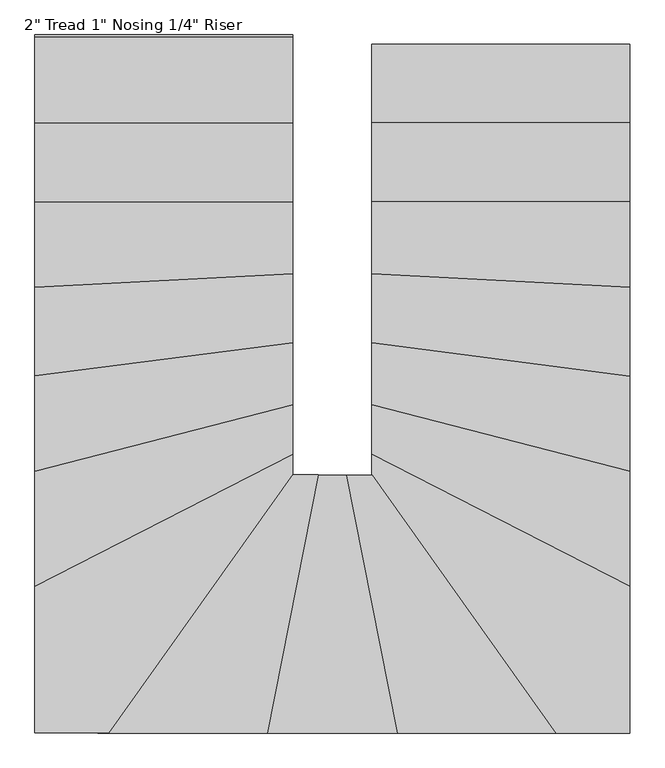
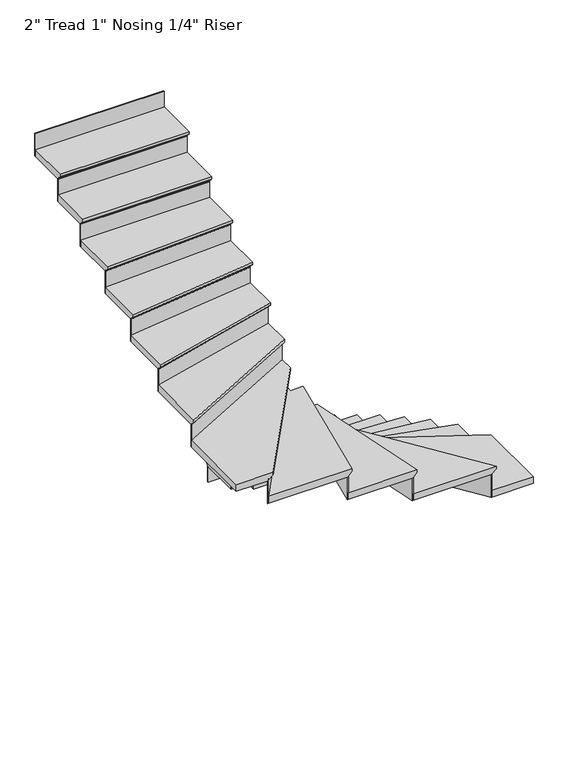
"""IFC4 building model written with IfcOpenShell, lengths in millimetres: stair flight geometry."""

from ifc_helpers import new_model, si_unit, origin, place, context, project, spatial, faceted_brep, source, transform, mapped, element, save


def stair_flight_703d0d0a(model_context):
    return source(origin(), model_context, "Body", "Brep", [
        faceted_brep([(-4178.4918623, -2804.4089531, 150.2833333), (-4178.4918623, -2804.4089531, 169.3333333), (-3264.0918623, -2804.4089531, 169.3333333), (-3264.0918623, -2804.4089531, 150.2833333), (-4178.4918623, -2829.8089531, 124.8833333), (-3264.0918623, -2829.8089531, 124.8833333), (-4178.4918623, -3109.2089531, 169.3333333), (-3264.0918623, -3109.2089531, 169.3333333), (-3264.0918623, -2829.8089531, 118.5333333), (-3264.0918623, -3109.2089531, 118.5333333), (-4178.4918623, -3109.2089531, 118.5333333), (-4178.4918623, -2829.8089531, 118.5333333)], [[[0, 1, 2, 3]], [[4, 0, 3, 5]], [[2, 1, 6, 7]], [[8, 9, 10, 11]], [[2, 7, 9, 8, 5, 3]], [[8, 11, 4, 5]], [[6, 1, 0, 4, 11, 10]], [[7, 6, 10, 9]]]),
        faceted_brep([(-4178.4918623, -2829.8089531, 118.5333333), (-4178.4918623, -2829.8089531, 0.0), (-4178.4918623, -2836.1589531, 0.0), (-4178.4918623, -2836.1589531, 118.5333333), (-3264.0918623, -2829.8089531, 118.5333333), (-3264.0918623, -2836.1589531, 118.5333333), (-3264.0918623, -2836.1589531, 0.0), (-3264.0918623, -2829.8089531, 0.0)], [[[0, 1, 2, 3]], [[4, 5, 6, 7]], [[1, 0, 4, 7]], [[2, 1, 7, 6]], [[3, 2, 6, 5]], [[0, 3, 5, 4]]]),
        faceted_brep([(-4178.4918623, -3109.2089531, 287.8666667), (-4178.4918623, -3109.2089531, 118.5333333), (-4178.4918623, -3115.5589531, 118.5333333), (-4178.4918623, -3115.5589531, 287.8666667), (-3264.0918623, -3109.2089531, 287.8666667), (-3264.0918623, -3115.5589531, 287.8666667), (-3264.0918623, -3115.5589531, 118.5333333), (-3264.0918623, -3109.2089531, 118.5333333)], [[[0, 1, 2, 3]], [[4, 5, 6, 7]], [[1, 0, 4, 7]], [[2, 1, 7, 6]], [[3, 2, 6, 5]], [[0, 3, 5, 4]]]),
        faceted_brep([(-3264.0918623, -3083.8089531, 338.6666667), (-4178.4918623, -3083.8089531, 338.6666667), (-4178.4918623, -3388.6089531, 338.6666667), (-3264.0918623, -3388.6089531, 338.6666667), (-3264.0918623, -3109.2089531, 287.8666667), (-3264.0918623, -3388.6089531, 287.8666667), (-4178.4918623, -3388.6089531, 287.8666667), (-4178.4918623, -3109.2089531, 287.8666667), (-3264.0918623, -3109.2089531, 294.2166667), (-3264.0918623, -3083.8089531, 319.6166667), (-4178.4918623, -3109.2089531, 294.2166667), (-4178.4918623, -3083.8089531, 319.6166667)], [[[0, 1, 2, 3]], [[4, 5, 6, 7]], [[0, 3, 5, 4, 8, 9]], [[4, 7, 10, 8]], [[2, 1, 11, 10, 7, 6]], [[3, 2, 6, 5]], [[11, 1, 0, 9]], [[10, 11, 9, 8]]]),
        faceted_brep([(-4178.4918623, -3388.6089531, 457.2), (-4178.4918623, -3388.6089531, 287.8666667), (-4178.4918623, -3394.9589531, 287.8666667), (-4178.4918623, -3394.9589531, 457.2), (-3264.0918623, -3388.6089531, 457.2), (-3264.0918623, -3394.9589531, 457.2), (-3264.0918623, -3394.9589531, 287.8666667), (-3264.0918623, -3388.6089531, 287.8666667)], [[[0, 1, 2, 3]], [[4, 5, 6, 7]], [[1, 0, 4, 7]], [[2, 1, 7, 6]], [[3, 2, 6, 5]], [[0, 3, 5, 4]]]),
        faceted_brep([(-3264.0918623, -3363.2089531, 508.0), (-4178.4918623, -3363.2089531, 508.0), (-4178.4918623, -3644.2761146, 508.0), (-3264.0918623, -3691.810385, 508.0), (-3264.0918623, -3388.6089531, 457.2), (-3264.0918623, -3691.810385, 457.2), (-4178.4918623, -3644.2761146, 457.2), (-4178.4918623, -3388.6089531, 457.2), (-3264.0918623, -3388.6089531, 463.55), (-3264.0918623, -3363.2089531, 488.95), (-4178.4918623, -3388.6089531, 463.55), (-4178.4918623, -3363.2089531, 488.95)], [[[0, 1, 2, 3]], [[4, 5, 6, 7]], [[0, 3, 5, 4, 8, 9]], [[4, 7, 10, 8]], [[2, 1, 11, 10, 7, 6]], [[3, 2, 6, 5]], [[11, 1, 0, 9]], [[10, 11, 9, 8]]]),
        faceted_brep([(-4178.4918623, -3644.2761146, 626.5333333), (-4178.4918623, -3644.2761146, 457.2), (-4178.4918623, -3650.6346887, 457.2), (-4178.4918623, -3650.6346887, 626.5333333), (-3264.0918623, -3691.810385, 626.5333333), (-3264.0918623, -3698.1689591, 626.5333333), (-3264.0918623, -3698.1689591, 457.2), (-3264.0918623, -3691.810385, 457.2)], [[[0, 1, 2, 3]], [[4, 5, 6, 7]], [[1, 0, 4, 7]], [[2, 1, 7, 6]], [[3, 2, 6, 5]], [[0, 3, 5, 4]]]),
        faceted_brep([(-3264.0918623, -3666.3760883, 677.3333333), (-4178.4918623, -3618.8418179, 677.3333333), (-4178.4918623, -3888.4428144, 677.3333333), (-3264.0918623, -4006.798866, 677.3333333), (-3264.0918623, -3691.810385, 626.5333333), (-3264.0918623, -4006.798866, 626.5333333), (-4178.4918623, -3888.4428144, 626.5333333), (-4178.4918623, -3644.2761146, 626.5333333), (-3264.0918623, -3691.810385, 632.8833333), (-3264.0918623, -3666.3760883, 658.2833333), (-4178.4918623, -3644.2761146, 632.8833333), (-4178.4918623, -3618.8418179, 658.2833333)], [[[0, 1, 2, 3]], [[4, 5, 6, 7]], [[0, 3, 5, 4, 8, 9]], [[4, 7, 10, 8]], [[2, 1, 11, 10, 7, 6]], [[3, 2, 6, 5]], [[11, 1, 0, 9]], [[10, 11, 9, 8]]]),
        faceted_brep([(-4178.4918623, -3888.4428144, 795.8666667), (-4178.4918623, -3888.4428144, 626.5333333), (-4178.4918623, -3894.8457862, 626.5333333), (-4178.4918623, -3894.8457862, 795.8666667), (-3264.0918623, -4006.798866, 795.8666667), (-3264.0918623, -4013.2018378, 795.8666667), (-3264.0918623, -4013.2018378, 626.5333333), (-3264.0918623, -4006.798866, 626.5333333)], [[[0, 1, 2, 3]], [[4, 5, 6, 7]], [[1, 0, 4, 7]], [[2, 1, 7, 6]], [[3, 2, 6, 5]], [[0, 3, 5, 4]]]),
        faceted_brep([(-3264.0918623, -3981.1869789, 846.6666667), (-4178.4918623, -3862.8309273, 846.6666667), (-4178.4918623, -4110.0700369, 846.6666667), (-3264.0918623, -4345.2004843, 846.6666667), (-3264.0918623, -4006.798866, 795.8666667), (-3264.0918623, -4345.2004843, 795.8666667), (-4178.4918623, -4110.0700369, 795.8666667), (-4178.4918623, -3888.4428144, 795.8666667), (-3264.0918623, -4006.798866, 802.2166667), (-3264.0918623, -3981.1869789, 827.6166667), (-4178.4918623, -3888.4428144, 802.2166667), (-4178.4918623, -3862.8309273, 827.6166667)], [[[0, 1, 2, 3]], [[4, 5, 6, 7]], [[0, 3, 5, 4, 8, 9]], [[4, 7, 10, 8]], [[2, 1, 11, 10, 7, 6]], [[3, 2, 6, 5]], [[11, 1, 0, 9]], [[10, 11, 9, 8]]]),
        faceted_brep([(-4178.4918623, -4110.0700369, 965.2), (-4178.4918623, -4110.0700369, 795.8666667), (-4178.4918623, -4116.6266137, 795.8666667), (-4178.4918623, -4116.6266137, 965.2), (-3264.0918623, -4345.2004843, 965.2), (-3264.0918623, -4351.7570611, 965.2), (-3264.0918623, -4351.7570611, 795.8666667), (-3264.0918623, -4345.2004843, 795.8666667)], [[[0, 1, 2, 3]], [[4, 5, 6, 7]], [[1, 0, 4, 7]], [[2, 1, 7, 6]], [[3, 2, 6, 5]], [[0, 3, 5, 4]]]),
        faceted_brep([(-3264.0918623, -4318.9741768, 1016.0), (-4178.4918623, -4083.8437294, 1016.0), (-4178.4918623, -4286.4166729, 1016.0), (-3264.0918623, -4755.2412943, 1016.0), (-3264.0918623, -4345.2004843, 965.2), (-3264.0918623, -4755.2412943, 965.2), (-4178.4918623, -4286.4166729, 965.2), (-4178.4918623, -4110.0700369, 965.2), (-3264.0918623, -4345.2004843, 971.55), (-3264.0918623, -4318.9741768, 996.95), (-4178.4918623, -4110.0700369, 971.55), (-4178.4918623, -4083.8437294, 996.95)], [[[0, 1, 2, 3]], [[4, 5, 6, 7]], [[0, 3, 5, 4, 8, 9]], [[4, 7, 10, 8]], [[2, 1, 11, 10, 7, 6]], [[3, 2, 6, 5]], [[11, 1, 0, 9]], [[10, 11, 9, 8]]]),
        faceted_brep([(-4178.4918623, -4286.4166729, 1134.5333333), (-4178.4918623, -4286.4166729, 965.2), (-4178.4918623, -4293.5526561, 965.2), (-4178.4918623, -4293.5526561, 1134.5333333), (-3264.0918623, -4755.2412943, 1134.5333333), (-3264.0918623, -4762.3772774, 1134.5333333), (-3264.0918623, -4762.3772774, 965.2), (-3264.0918623, -4755.2412943, 965.2)], [[[0, 1, 2, 3]], [[4, 5, 6, 7]], [[1, 0, 4, 7]], [[2, 1, 7, 6]], [[3, 2, 6, 5]], [[0, 3, 5, 4]]]),
        faceted_brep([(-3557.772996, -5246.540645, 1185.3333333), (-3264.0918623, -5246.540645, 1185.3333333), (-3264.0918623, -4726.6973617, 1185.3333333), (-4178.4918623, -4257.8727404, 1185.3333333), (-4178.4918623, -4332.140645, 1185.3333333), (-4208.0469452, -4332.140645, 1185.3333333), (-3264.0918623, -5246.540645, 1134.5333333), (-3557.772996, -5246.540645, 1134.5333333), (-4208.0469452, -4332.140645, 1134.5333333), (-4178.4918623, -4332.140645, 1134.5333333), (-4178.4918623, -4286.4166729, 1134.5333333), (-3264.0918623, -4755.2412943, 1134.5333333), (-3264.0918623, -4755.2412943, 1140.8833333), (-3264.0918623, -4726.6973617, 1166.2833333), (-4178.4918623, -4286.4166729, 1140.8833333), (-4178.4918623, -4257.8727404, 1166.2833333)], [[[0, 1, 2, 3, 4, 5]], [[6, 7, 8, 9, 10, 11]], [[1, 0, 7, 6]], [[2, 1, 6, 11, 12, 13]], [[11, 10, 14, 12]], [[4, 3, 15, 14, 10, 9]], [[5, 4, 9, 8]], [[0, 5, 8, 7]], [[15, 3, 2, 13]], [[14, 15, 13, 12]]]),
        faceted_brep([(-4208.0469452, -4332.140645, 1303.8666667), (-4208.0469452, -4332.140645, 1134.5333333), (-4215.83892, -4332.140645, 1134.5333333), (-4215.83892, -4332.140645, 1303.8666667), (-3557.772996, -5246.540645, 1303.8666667), (-3565.5649708, -5246.540645, 1303.8666667), (-3565.5649708, -5246.540645, 1134.5333333), (-3557.772996, -5246.540645, 1134.5333333)], [[[0, 1, 2, 3]], [[4, 5, 6, 7]], [[1, 0, 4, 7]], [[2, 1, 7, 6]], [[3, 2, 6, 5]], [[0, 3, 5, 4]]]),
        faceted_brep([(-3526.6050968, -5246.540645, 1354.6666667), (-4176.879046, -4332.140645, 1354.6666667), (-4294.5010322, -4332.140645, 1354.6666667), (-4114.2601759, -5246.540645, 1354.6666667), (-3557.772996, -5246.540645, 1303.8666667), (-4114.2601759, -5246.540645, 1303.8666667), (-4294.5010322, -4332.140645, 1303.8666667), (-4208.0469452, -4332.140645, 1303.8666667), (-3557.772996, -5246.540645, 1310.2166667), (-3526.6050968, -5246.540645, 1335.6166667), (-4208.0469452, -4332.140645, 1310.2166667), (-4176.879046, -4332.140645, 1335.6166667)], [[[0, 1, 2, 3]], [[4, 5, 6, 7]], [[0, 3, 5, 4, 8, 9]], [[4, 7, 10, 8]], [[2, 1, 11, 10, 7, 6]], [[3, 2, 6, 5]], [[11, 1, 0, 9]], [[10, 11, 9, 8]]]),
        faceted_brep([(-4294.5010322, -4332.140645, 1473.2), (-4294.5010322, -4332.140645, 1303.8666667), (-4300.9732177, -4332.140645, 1303.8666667), (-4300.9732177, -4332.140645, 1473.2), (-4114.2601759, -5246.540645, 1473.2), (-4120.7323613, -5246.540645, 1473.2), (-4120.7323613, -5246.540645, 1303.8666667), (-4114.2601759, -5246.540645, 1303.8666667)], [[[0, 1, 2, 3]], [[4, 5, 6, 7]], [[1, 0, 4, 7]], [[2, 1, 7, 6]], [[3, 2, 6, 5]], [[0, 3, 5, 4]]]),
        faceted_brep([(-4088.3714342, -5246.540645, 1524.0), (-4268.6122905, -4332.140645, 1524.0), (-4393.6601759, -4332.140645, 1524.0), (-4573.9010322, -5246.540645, 1524.0), (-4114.2601759, -5246.540645, 1473.2), (-4573.9010322, -5246.540645, 1473.2), (-4393.6601759, -4332.140645, 1473.2), (-4294.5010322, -4332.140645, 1473.2), (-4114.2601759, -5246.540645, 1479.55), (-4088.3714342, -5246.540645, 1504.95), (-4294.5010322, -4332.140645, 1479.55), (-4268.6122905, -4332.140645, 1504.95)], [[[0, 1, 2, 3]], [[4, 5, 6, 7]], [[0, 3, 5, 4, 8, 9]], [[4, 7, 10, 8]], [[2, 1, 11, 10, 7, 6]], [[3, 2, 6, 5]], [[11, 1, 0, 9]], [[10, 11, 9, 8]]]),
        faceted_brep([(-4393.6601759, -4332.140645, 1642.5333333), (-4393.6601759, -4332.140645, 1473.2), (-4400.1323613, -4332.140645, 1473.2), (-4400.1323613, -4332.140645, 1642.5333333), (-4573.9010322, -5246.540645, 1642.5333333), (-4580.3732177, -5246.540645, 1642.5333333), (-4580.3732177, -5246.540645, 1473.2), (-4573.9010322, -5246.540645, 1473.2)], [[[0, 1, 2, 3]], [[4, 5, 6, 7]], [[1, 0, 4, 7]], [[2, 1, 7, 6]], [[3, 2, 6, 5]], [[0, 3, 5, 4]]]),
        faceted_brep([(-4548.0122905, -5246.540645, 1693.3333333), (-4367.7714342, -4332.140645, 1693.3333333), (-4457.8918623, -4332.140645, 1693.3333333), (-4457.8918623, -4286.0451704, 1693.3333333), (-5140.946527, -5246.540645, 1693.3333333), (-4573.9010322, -5246.540645, 1642.5333333), (-5140.946527, -5246.540645, 1642.5333333), (-4457.8918623, -4286.0451704, 1642.5333333), (-4457.8918623, -4332.140645, 1642.5333333), (-4393.6601759, -4332.140645, 1642.5333333), (-4573.9010322, -5246.540645, 1648.8833333), (-4548.0122905, -5246.540645, 1674.2833333), (-4393.6601759, -4332.140645, 1648.8833333), (-4367.7714342, -4332.140645, 1674.2833333)], [[[0, 1, 2, 3, 4]], [[5, 6, 7, 8, 9]], [[0, 4, 6, 5, 10, 11]], [[5, 9, 12, 10]], [[2, 1, 13, 12, 9, 8]], [[3, 2, 8, 7]], [[4, 3, 7, 6]], [[13, 1, 0, 11]], [[12, 13, 11, 10]]]),
        faceted_brep([(-4457.8918623, -4286.0451704, 1811.8666667), (-4457.8918623, -4286.0451704, 1642.5333333), (-4457.8918623, -4275.0882779, 1642.5333333), (-4457.8918623, -4275.0882779, 1811.8666667), (-5140.946527, -5246.540645, 1811.8666667), (-5148.7385018, -5246.540645, 1811.8666667), (-5148.7385018, -5246.540645, 1642.5333333), (-5140.946527, -5246.540645, 1642.5333333)], [[[0, 1, 2, 3]], [[4, 5, 6, 7]], [[1, 0, 4, 7]], [[2, 1, 7, 6]], [[3, 2, 6, 5]], [[0, 3, 5, 4]]]),
        faceted_brep([(-5372.2918623, -4698.1534292, 1862.6666667), (-5372.2918623, -5246.540645, 1862.6666667), (-5109.7786278, -5246.540645, 1862.6666667), (-4457.8918623, -4329.8727404, 1862.6666667), (-4457.8918623, -4229.3288079, 1862.6666667), (-5372.2918623, -5246.540645, 1811.8666667), (-5372.2918623, -4698.1534292, 1811.8666667), (-4457.8918623, -4229.3288079, 1811.8666667), (-4457.8918623, -4286.0451704, 1811.8666667), (-5140.946527, -5246.540645, 1811.8666667), (-5140.946527, -5246.540645, 1818.2166667), (-5109.7786278, -5246.540645, 1843.6166667), (-4457.8918623, -4286.0451704, 1818.2166667), (-4457.8918623, -4329.8727404, 1843.6166667)], [[[0, 1, 2, 3, 4]], [[5, 6, 7, 8, 9]], [[1, 0, 6, 5]], [[2, 1, 5, 9, 10, 11]], [[9, 8, 12, 10]], [[4, 3, 13, 12, 8, 7]], [[0, 4, 7, 6]], [[13, 3, 2, 11]], [[12, 13, 11, 10]]]),
        faceted_brep([(-4457.8918623, -4229.3288079, 1981.2), (-4457.8918623, -4229.3288079, 1811.8666667), (-4457.8918623, -4222.1928247, 1811.8666667), (-4457.8918623, -4222.1928247, 1981.2), (-5372.2918623, -4698.1534292, 1981.2), (-5372.2918623, -4691.0174461, 1981.2), (-5372.2918623, -4691.0174461, 1811.8666667), (-5372.2918623, -4698.1534292, 1811.8666667)], [[[0, 1, 2, 3]], [[4, 5, 6, 7]], [[1, 0, 4, 7]], [[2, 1, 7, 6]], [[3, 2, 6, 5]], [[0, 3, 5, 4]]]),
        faceted_brep([(-5372.2918623, -4726.6973617, 2032.0), (-4457.8918623, -4257.8727404, 2032.0), (-4457.8918623, -4057.6174219, 2032.0), (-5372.2918623, -4292.7478693, 2032.0), (-5372.2918623, -4698.1534292, 1981.2), (-5372.2918623, -4292.7478693, 1981.2), (-4457.8918623, -4057.6174219, 1981.2), (-4457.8918623, -4229.3288079, 1981.2), (-5372.2918623, -4698.1534292, 1987.55), (-5372.2918623, -4726.6973617, 2012.95), (-4457.8918623, -4229.3288079, 1987.55), (-4457.8918623, -4257.8727404, 2012.95)], [[[0, 1, 2, 3]], [[4, 5, 6, 7]], [[0, 3, 5, 4, 8, 9]], [[4, 7, 10, 8]], [[2, 1, 11, 10, 7, 6]], [[3, 2, 6, 5]], [[11, 1, 0, 9]], [[10, 11, 9, 8]]]),
        faceted_brep([(-4457.8918623, -4057.6174219, 2150.5333333), (-4457.8918623, -4057.6174219, 1981.2), (-4457.8918623, -4051.0608451, 1981.2), (-4457.8918623, -4051.0608451, 2150.5333333), (-5372.2918623, -4292.7478693, 2150.5333333), (-5372.2918623, -4286.1912925, 2150.5333333), (-5372.2918623, -4286.1912925, 1981.2), (-5372.2918623, -4292.7478693, 1981.2)], [[[0, 1, 2, 3]], [[4, 5, 6, 7]], [[1, 0, 4, 7]], [[2, 1, 7, 6]], [[3, 2, 6, 5]], [[0, 3, 5, 4]]]),
        faceted_brep([(-5372.2918623, -4318.9741768, 2201.3333333), (-4457.8918623, -4083.8437294, 2201.3333333), (-4457.8918623, -3837.2190402, 2201.3333333), (-5372.2918623, -3955.5750918, 2201.3333333), (-5372.2918623, -4292.7478693, 2150.5333333), (-5372.2918623, -3955.5750918, 2150.5333333), (-4457.8918623, -3837.2190402, 2150.5333333), (-4457.8918623, -4057.6174219, 2150.5333333), (-5372.2918623, -4292.7478693, 2156.8833333), (-5372.2918623, -4318.9741768, 2182.2833333), (-4457.8918623, -4057.6174219, 2156.8833333), (-4457.8918623, -4083.8437294, 2182.2833333)], [[[0, 1, 2, 3]], [[4, 5, 6, 7]], [[0, 3, 5, 4, 8, 9]], [[4, 7, 10, 8]], [[2, 1, 11, 10, 7, 6]], [[3, 2, 6, 5]], [[11, 1, 0, 9]], [[10, 11, 9, 8]]]),
        faceted_brep([(-4457.8918623, -3837.2190402, 2319.8666667), (-4457.8918623, -3837.2190402, 2150.5333333), (-4457.8918623, -3830.8160684, 2150.5333333), (-4457.8918623, -3830.8160684, 2319.8666667), (-5372.2918623, -3955.5750918, 2319.8666667), (-5372.2918623, -3949.17212, 2319.8666667), (-5372.2918623, -3949.17212, 2150.5333333), (-5372.2918623, -3955.5750918, 2150.5333333)], [[[0, 1, 2, 3]], [[4, 5, 6, 7]], [[1, 0, 4, 7]], [[2, 1, 7, 6]], [[3, 2, 6, 5]], [[0, 3, 5, 4]]]),
        faceted_brep([(-5372.2918623, -3981.1869789, 2370.6666667), (-4457.8918623, -3862.8309273, 2370.6666667), (-4457.8918623, -3593.4075212, 2370.6666667), (-5372.2918623, -3640.9417916, 2370.6666667), (-5372.2918623, -3955.5750918, 2319.8666667), (-5372.2918623, -3640.9417916, 2319.8666667), (-4457.8918623, -3593.4075212, 2319.8666667), (-4457.8918623, -3837.2190402, 2319.8666667), (-5372.2918623, -3955.5750918, 2326.2166667), (-5372.2918623, -3981.1869789, 2351.6166667), (-4457.8918623, -3837.2190402, 2326.2166667), (-4457.8918623, -3862.8309273, 2351.6166667)], [[[0, 1, 2, 3]], [[4, 5, 6, 7]], [[0, 3, 5, 4, 8, 9]], [[4, 7, 10, 8]], [[2, 1, 11, 10, 7, 6]], [[3, 2, 6, 5]], [[11, 1, 0, 9]], [[10, 11, 9, 8]]]),
        faceted_brep([(-4457.8918623, -3593.4075212, 2489.2), (-4457.8918623, -3593.4075212, 2319.8666667), (-4457.8918623, -3587.0489471, 2319.8666667), (-4457.8918623, -3587.0489471, 2489.2), (-5372.2918623, -3640.9417916, 2489.2), (-5372.2918623, -3634.5832175, 2489.2), (-5372.2918623, -3634.5832175, 2319.8666667), (-5372.2918623, -3640.9417916, 2319.8666667)], [[[0, 1, 2, 3]], [[4, 5, 6, 7]], [[1, 0, 4, 7]], [[2, 1, 7, 6]], [[3, 2, 6, 5]], [[0, 3, 5, 4]]]),
        faceted_brep([(-5372.2918623, -3666.3760883, 2540.0), (-4457.8918623, -3618.8418179, 2540.0), (-4457.8918623, -3337.8089531, 2540.0), (-5372.2918623, -3337.8089531, 2540.0), (-5372.2918623, -3640.9417916, 2489.2), (-5372.2918623, -3337.8089531, 2489.2), (-4457.8918623, -3337.8089531, 2489.2), (-4457.8918623, -3593.4075212, 2489.2), (-5372.2918623, -3640.9417916, 2495.55), (-5372.2918623, -3666.3760883, 2520.95), (-4457.8918623, -3593.4075212, 2495.55), (-4457.8918623, -3618.8418179, 2520.95)], [[[0, 1, 2, 3]], [[4, 5, 6, 7]], [[0, 3, 5, 4, 8, 9]], [[4, 7, 10, 8]], [[2, 1, 11, 10, 7, 6]], [[3, 2, 6, 5]], [[11, 1, 0, 9]], [[10, 11, 9, 8]]]),
        faceted_brep([(-4457.8918623, -3337.8089531, 2658.5333333), (-4457.8918623, -3337.8089531, 2489.2), (-4457.8918623, -3331.4589531, 2489.2), (-4457.8918623, -3331.4589531, 2658.5333333), (-5372.2918623, -3337.8089531, 2658.5333333), (-5372.2918623, -3331.4589531, 2658.5333333), (-5372.2918623, -3331.4589531, 2489.2), (-5372.2918623, -3337.8089531, 2489.2)], [[[0, 1, 2, 3]], [[4, 5, 6, 7]], [[1, 0, 4, 7]], [[2, 1, 7, 6]], [[3, 2, 6, 5]], [[0, 3, 5, 4]]]),
        faceted_brep([(-5372.2918623, -3363.2089531, 2709.3333333), (-4457.8918623, -3363.2089531, 2709.3333333), (-4457.8918623, -3058.4089531, 2709.3333333), (-5372.2918623, -3058.4089531, 2709.3333333), (-5372.2918623, -3337.8089531, 2658.5333333), (-5372.2918623, -3058.4089531, 2658.5333333), (-4457.8918623, -3058.4089531, 2658.5333333), (-4457.8918623, -3337.8089531, 2658.5333333), (-5372.2918623, -3337.8089531, 2664.8833333), (-5372.2918623, -3363.2089531, 2690.2833333), (-4457.8918623, -3337.8089531, 2664.8833333), (-4457.8918623, -3363.2089531, 2690.2833333)], [[[0, 1, 2, 3]], [[4, 5, 6, 7]], [[0, 3, 5, 4, 8, 9]], [[4, 7, 10, 8]], [[2, 1, 11, 10, 7, 6]], [[3, 2, 6, 5]], [[11, 1, 0, 9]], [[10, 11, 9, 8]]]),
        faceted_brep([(-4457.8918623, -3058.4089531, 2827.8666667), (-4457.8918623, -3058.4089531, 2658.5333333), (-4457.8918623, -3052.0589531, 2658.5333333), (-4457.8918623, -3052.0589531, 2827.8666667), (-5372.2918623, -3058.4089531, 2827.8666667), (-5372.2918623, -3052.0589531, 2827.8666667), (-5372.2918623, -3052.0589531, 2658.5333333), (-5372.2918623, -3058.4089531, 2658.5333333)], [[[0, 1, 2, 3]], [[4, 5, 6, 7]], [[1, 0, 4, 7]], [[2, 1, 7, 6]], [[3, 2, 6, 5]], [[0, 3, 5, 4]]]),
        faceted_brep([(-4457.8918623, -2779.0089531, 2997.2), (-4457.8918623, -2779.0089531, 2827.8666667), (-4457.8918623, -2772.6589531, 2827.8666667), (-4457.8918623, -2772.6589531, 2997.2), (-5372.2918623, -2779.0089531, 2997.2), (-5372.2918623, -2772.6589531, 2997.2), (-5372.2918623, -2772.6589531, 2827.8666667), (-5372.2918623, -2779.0089531, 2827.8666667)], [[[0, 1, 2, 3]], [[4, 5, 6, 7]], [[1, 0, 4, 7]], [[2, 1, 7, 6]], [[3, 2, 6, 5]], [[0, 3, 5, 4]]]),
        faceted_brep([(-5372.2918623, -3083.8089531, 2878.6666667), (-4457.8918623, -3083.8089531, 2878.6666667), (-4457.8918623, -2779.0089531, 2878.6666667), (-5372.2918623, -2779.0089531, 2878.6666667), (-5372.2918623, -3058.4089531, 2827.8666667), (-5372.2918623, -2779.0089531, 2827.8666667), (-4457.8918623, -2779.0089531, 2827.8666667), (-4457.8918623, -3058.4089531, 2827.8666667), (-5372.2918623, -3058.4089531, 2834.2166667), (-5372.2918623, -3083.8089531, 2859.6166667), (-4457.8918623, -3058.4089531, 2834.2166667), (-4457.8918623, -3083.8089531, 2859.6166667)], [[[0, 1, 2, 3]], [[4, 5, 6, 7]], [[0, 3, 5, 4, 8, 9]], [[4, 7, 10, 8]], [[2, 1, 11, 10, 7, 6]], [[3, 2, 6, 5]], [[11, 1, 0, 9]], [[10, 11, 9, 8]]]),
    ])


if __name__ == "__main__":
    model = new_model("IFC4")
    model_context = context("Model", 3, world=origin())
    ifc_project = project(units=[si_unit("LENGTHUNIT", "METRE", prefix="MILLI")], contexts=[model_context])
    site = spatial("IfcSite", under=ifc_project)
    building = spatial("IfcBuilding", under=site)
    placement = place(None, origin())
    stair_flight_shape = stair_flight_703d0d0a(model_context)
    element("IfcStairFlight", 1, ObjectType="2\" Tread 1\" Nosing 1/4\" Riser", at=placement, inside=building, context=model_context, shape_type="MappedRepresentation", body=[
        mapped(stair_flight_shape, transform((0.0, 0.0, 0.0), x_axis=(1.0, 0.0, 0.0), y_axis=(0.0, 1.0, 0.0), z_axis=(0.0, 0.0, 1.0))),
    ])
    save(model, "model.ifc")
